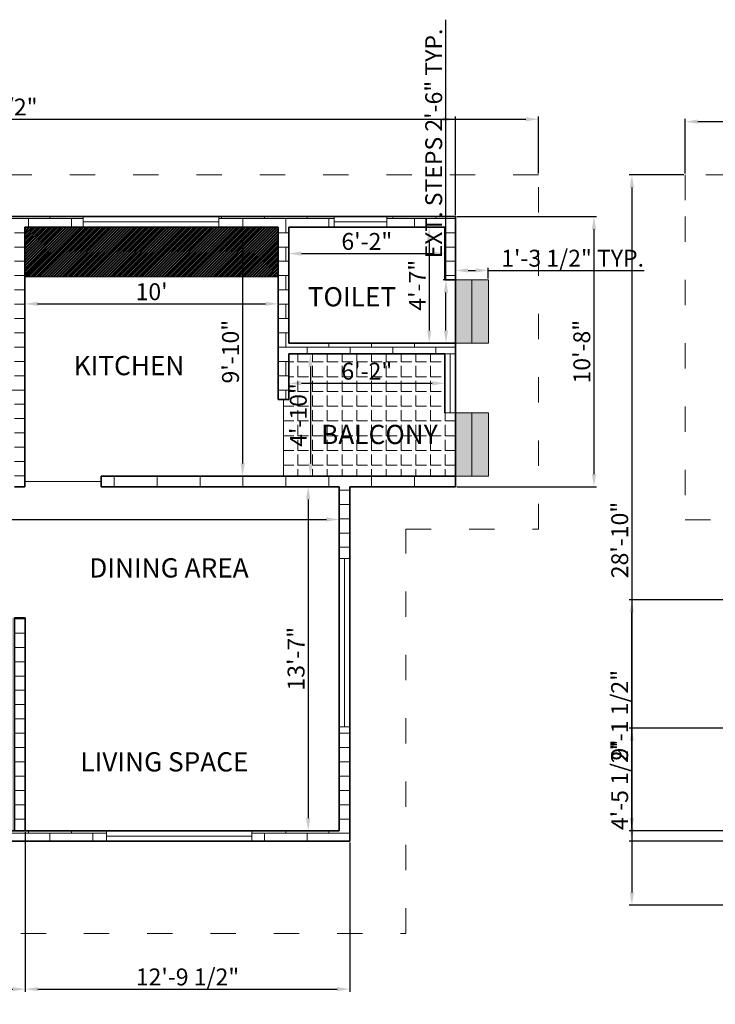
# Model space of a CAD drawing. Units: millimetres. Extents: x 1518 to 2850, y 936 to 2174.
# Tile 3 of 5: x 2007 to 2336, y 1707 to 2174. Entities that reach past the tile are written whole.
import ezdxf

# ---------------------------------------------------------------- set-up
doc = ezdxf.new("R2010")
doc.units = ezdxf.units.MM
doc.linetypes.add('ACAD_ISO03W100', pattern=[30, 12, -18])
for name, color, linetype, lineweight, true_color in [('A-ANNO-DIMS', 9, 'Continuous', 18, 0xafd9aa), ('A-AREA-IDEN', 31, 'Continuous', 18, 0xfecc66), ('A-DOOR', 244, 'Continuous', 20, 0x991b1e), ('A-FLOR-FIXT-PATT', 254, 'Continuous', 13, 0xfeeab9), ('A-FLOR-PATT', 252, 'Continuous', 13, 0x939598), ('A-GLAZ', 141, 'Continuous', 18, 0xadddf7), ('A-ROOF-OVHD', 177, 'ACAD_ISO03W100', 18, 0x293189)]:
    doc.layers.add(name, color=color, linetype=linetype, lineweight=lineweight, true_color=true_color)
for name, color, linetype, lineweight in [('A-FLOR-FIXT', 8, 'Continuous', 18), ('A-FLOR-STRS', 7, 'Continuous', 20), ('A-FLOR-STRS-PATT', 7, 'Continuous', 13), ('A-WALL', 7, 'Continuous', 35), ('A-WALL-PATT', 7, 'Continuous', 13)]:
    doc.layers.add(name, color=color, linetype=linetype, lineweight=lineweight)
doc.styles.get("Standard").update_dxf_attribs({"font": 'arial.ttf'})
doc.dimstyles.new('ISO-25', dxfattribs={"dimtxt": 8, "dimasz": 6, "dimexe": 1.25, "dimexo": 0.625, "dimtad": 1, "dimdec": 0, "dimlunit": 3, "dimtxsty": 'Standard', "dimcen": 2.5, "dimadec": 0, "dimazin": 0, "dimtfac": 1, "dimtdec": 0, "dimtmove": 0, "dimatfit": 3, "dimfxl": 1, "dimarcsym": 0})

# ---------------------------------------------------------------- blocks, each defined once
blk = doc.blocks.new('*D5')
at = {"layer": 'A-ANNO-DIMS', "color": 0, "lineweight": -2, "transparency": 16777216}
for p, q in [((1790.95, 1951.97), (1790.95, 1935.8)), ((2158.01, 1951.97), (2158.01, 1935.8)), ((1796.95, 1937.05), (2152.01, 1937.05))]:
    blk.add_line(p, q, dxfattribs=at)
at = {"layer": 'A-ANNO-DIMS', "color": 0, "transparency": 16777216}
for points in [[(1796.95, 1938.05), (1796.95, 1936.05), (1790.95, 1937.05)], [(2152.01, 1938.05), (2152.01, 1936.05), (2158.01, 1937.05)]]:
    blk.add_solid(points, dxfattribs=at)
at = {"layer": 'Defpoints', "color": 0, "transparency": 16777216}
for p in [(1790.95, 1952.6), (2158.01, 1952.6), (2158.01, 1937.05)]:
    blk.add_point(p, dxfattribs=at)
at = {"layer": 'A-ANNO-DIMS', "color": 0, "transparency": 16777216, "insert": (1974.48, 1941.76), "char_height": 8, "attachment_point": 5}
blk.add_mtext('30\'-7"', dxfattribs=at)
blk = doc.blocks.new('*D7')
at = {"layer": 'A-ANNO-DIMS', "color": 0, "lineweight": -2, "transparency": 16777216}
for p, q in [((2009.13, 2074.9), (2009.13, 2037.95)), ((2129.13, 2074.9), (2129.13, 2037.95)), ((2015.13, 2039.2), (2123.13, 2039.2))]:
    blk.add_line(p, q, dxfattribs=at)
at = {"layer": 'A-ANNO-DIMS', "color": 0, "transparency": 16777216}
for points in [[(2015.13, 2040.2), (2015.13, 2038.2), (2009.13, 2039.2)], [(2123.13, 2040.2), (2123.13, 2038.2), (2129.13, 2039.2)]]:
    blk.add_solid(points, dxfattribs=at)
at = {"layer": 'Defpoints', "color": 0, "transparency": 16777216}
for p in [(2009.13, 2075.52), (2129.13, 2075.52), (2129.13, 2039.2)]:
    blk.add_point(p, dxfattribs=at)
at = {"layer": 'A-ANNO-DIMS', "color": 0, "transparency": 16777216, "insert": (2069.13, 2043.91), "char_height": 8, "attachment_point": 5}
blk.add_mtext("10'", dxfattribs=at)
blk = doc.blocks.new('*D8')
at = {"layer": 'A-ANNO-DIMS', "color": 0, "lineweight": -2, "transparency": 16777216}
for p, q in [((2128.5, 2075.52), (2111.02, 2075.52)), ((2112.27, 2069.52), (2112.27, 1963.6)), ((2128.5, 1957.6), (2111.02, 1957.6))]:
    blk.add_line(p, q, dxfattribs=at)
at = {"layer": 'A-ANNO-DIMS', "color": 0, "transparency": 16777216}
for points in [[(2111.27, 2069.52), (2113.27, 2069.52), (2112.27, 2075.52)], [(2111.27, 1963.6), (2113.27, 1963.6), (2112.27, 1957.6)]]:
    blk.add_solid(points, dxfattribs=at)
at = {"layer": 'Defpoints', "color": 0, "transparency": 16777216}
for p in [(2129.13, 2075.52), (2112.27, 1957.6), (2129.13, 1957.6)]:
    blk.add_point(p, dxfattribs=at)
at = {"layer": 'A-ANNO-DIMS', "color": 0, "transparency": 16777216, "insert": (2107.56, 2016.56), "char_height": 8, "attachment_point": 5, "rotation": 90}
blk.add_mtext('9\'-10"', dxfattribs=at)
blk = doc.blocks.new('*D9')
at = {"layer": 'A-ANNO-DIMS', "color": 0, "lineweight": -2, "transparency": 16777216}
for p, q in [((2134.13, 2074.9), (2134.13, 2061.77)), ((2208.13, 2074.9), (2208.13, 2061.77)), ((2140.13, 2063.02), (2202.13, 2063.02))]:
    blk.add_line(p, q, dxfattribs=at)
at = {"layer": 'A-ANNO-DIMS', "color": 0, "transparency": 16777216}
for points in [[(2140.13, 2064.02), (2140.13, 2062.02), (2134.13, 2063.02)], [(2202.13, 2064.02), (2202.13, 2062.02), (2208.13, 2063.02)]]:
    blk.add_solid(points, dxfattribs=at)
at = {"layer": 'Defpoints', "color": 0, "transparency": 16777216}
for p in [(2134.13, 2075.52), (2208.13, 2075.52), (2208.13, 2063.02)]:
    blk.add_point(p, dxfattribs=at)
at = {"layer": 'A-ANNO-DIMS', "color": 0, "transparency": 16777216, "insert": (2171.13, 2067.73), "char_height": 8, "attachment_point": 5}
blk.add_mtext('6\'-2"', dxfattribs=at)
blk = doc.blocks.new('*D10')
at = {"layer": 'A-ANNO-DIMS', "color": 0, "lineweight": -2, "transparency": 16777216}
for p, q in [((2207.5, 2075.52), (2199.46, 2075.52)), ((2200.71, 2069.52), (2200.71, 2026.52)), ((2207.5, 2020.52), (2199.46, 2020.52))]:
    blk.add_line(p, q, dxfattribs=at)
at = {"layer": 'A-ANNO-DIMS', "color": 0, "transparency": 16777216}
for points in [[(2199.71, 2069.52), (2201.71, 2069.52), (2200.71, 2075.52)], [(2199.71, 2026.52), (2201.71, 2026.52), (2200.71, 2020.52)]]:
    blk.add_solid(points, dxfattribs=at)
at = {"layer": 'Defpoints', "color": 0, "transparency": 16777216}
for p in [(2208.13, 2075.52), (2200.71, 2020.52), (2208.13, 2020.52)]:
    blk.add_point(p, dxfattribs=at)
at = {"layer": 'A-ANNO-DIMS', "color": 0, "transparency": 16777216, "insert": (2196.09, 2048.02), "char_height": 8, "attachment_point": 5, "rotation": 90}
blk.add_mtext('4\'-7"', dxfattribs=at)
blk = doc.blocks.new('*D11')
at = {"layer": 'A-ANNO-DIMS', "color": 0, "lineweight": -2, "transparency": 16777216}
for p, q in [((2134.75, 2015.52), (2145.64, 2015.52)), ((2144.39, 2009.52), (2144.39, 1963.6)), ((2134.75, 1957.6), (2145.64, 1957.6))]:
    blk.add_line(p, q, dxfattribs=at)
at = {"layer": 'A-ANNO-DIMS', "color": 0, "transparency": 16777216}
for points in [[(2143.39, 2009.52), (2145.39, 2009.52), (2144.39, 2015.52)], [(2143.39, 1963.6), (2145.39, 1963.6), (2144.39, 1957.6)]]:
    blk.add_solid(points, dxfattribs=at)
at = {"layer": 'Defpoints', "color": 0, "transparency": 16777216}
for p in [(2134.13, 2015.52), (2134.13, 1957.6), (2144.39, 1957.6)]:
    blk.add_point(p, dxfattribs=at)
at = {"layer": 'A-ANNO-DIMS', "color": 0, "transparency": 16777216, "insert": (2139.68, 1986.56), "char_height": 8, "attachment_point": 5, "rotation": 90}
blk.add_mtext('4\'-10"', dxfattribs=at)
blk = doc.blocks.new('*D12')
at = {"layer": 'A-ANNO-DIMS', "color": 0, "lineweight": -2, "transparency": 16777216}
for p, q in [((2134.13, 2014.9), (2134.13, 2000.31)), ((2208.13, 2014.9), (2208.13, 2000.31)), ((2140.13, 2001.56), (2202.13, 2001.56))]:
    blk.add_line(p, q, dxfattribs=at)
at = {"layer": 'A-ANNO-DIMS', "color": 0, "transparency": 16777216}
for points in [[(2140.13, 2002.56), (2140.13, 2000.56), (2134.13, 2001.56)], [(2202.13, 2002.56), (2202.13, 2000.56), (2208.13, 2001.56)]]:
    blk.add_solid(points, dxfattribs=at)
at = {"layer": 'Defpoints', "color": 0, "transparency": 16777216}
for p in [(2134.13, 2015.52), (2208.13, 2015.52), (2208.13, 2001.56)]:
    blk.add_point(p, dxfattribs=at)
at = {"layer": 'A-ANNO-DIMS', "color": 0, "transparency": 16777216, "insert": (2171.13, 2006.27), "char_height": 8, "attachment_point": 5}
blk.add_mtext('6\'-2"', dxfattribs=at)
blk = doc.blocks.new('*D13')
at = {"layer": 'A-ANNO-DIMS', "color": 0, "lineweight": -2, "transparency": 16777216}
for p, q in [((2157.38, 1952.6), (2142.09, 1952.6)), ((2143.34, 1946.6), (2143.34, 1795.6)), ((2157.38, 1789.6), (2142.09, 1789.6))]:
    blk.add_line(p, q, dxfattribs=at)
at = {"layer": 'A-ANNO-DIMS', "color": 0, "transparency": 16777216}
for points in [[(2142.34, 1946.6), (2144.34, 1946.6), (2143.34, 1952.6)], [(2142.34, 1795.6), (2144.34, 1795.6), (2143.34, 1789.6)]]:
    blk.add_solid(points, dxfattribs=at)
at = {"layer": 'Defpoints', "color": 0, "transparency": 16777216}
for p in [(2158.01, 1952.6), (2143.34, 1789.6), (2158.01, 1789.6)]:
    blk.add_point(p, dxfattribs=at)
at = {"layer": 'A-ANNO-DIMS', "color": 0, "transparency": 16777216, "insert": (2138.63, 1871.1), "char_height": 8, "attachment_point": 5, "rotation": 90}
blk.add_mtext('13\'-7"', dxfattribs=at)
blk = doc.blocks.new('STEP-PAIR-EXT')
for points in [[(0, 30), (7.79, 30), (7.79, 0), (0, 0)], [(7.79, 30), (15.58, 30), (15.58, 0), (7.79, 0)]]:
    blk.add_lwpolyline(points, close=True)
blk = doc.blocks.new('*D28')
at = {"layer": 'A-ANNO-DIMS', "color": 0, "lineweight": -2, "transparency": 16777216}
for p, q in [((2208.63, 2050.52), (2208.63, 2173.81)), ((2212.5, 2050.52), (2207.38, 2050.52)), ((2208.63, 2026.52), (2208.63, 2044.52)), ((2212.5, 2020.52), (2207.38, 2020.52))]:
    blk.add_line(p, q, dxfattribs=at)
at = {"layer": 'A-ANNO-DIMS', "color": 0, "transparency": 16777216}
for points in [[(2207.63, 2044.52), (2209.63, 2044.52), (2208.63, 2050.52)], [(2207.63, 2026.52), (2209.63, 2026.52), (2208.63, 2020.52)]]:
    blk.add_solid(points, dxfattribs=at)
at = {"layer": 'Defpoints', "color": 0, "transparency": 16777216}
for p in [(2208.63, 2050.52), (2213.13, 2050.52), (2213.13, 2020.52)]:
    blk.add_point(p, dxfattribs=at)
at = {"layer": 'A-ANNO-DIMS', "color": 0, "transparency": 16777216, "insert": (2203.86, 2115.17), "char_height": 8, "attachment_point": 5, "rotation": 90}
blk.add_mtext('EXT. STEPS 2\'-6" TYP.', dxfattribs=at)
blk = doc.blocks.new('*D29')
at = {"layer": 'A-ANNO-DIMS', "color": 0, "lineweight": -2, "transparency": 16777216}
for p, q in [((2213.13, 2051.15), (2213.13, 2056.27)), ((2219.13, 2055.02), (2222.7, 2055.02)), ((2228.7, 2051.15), (2228.7, 2056.27)), ((2228.7, 2055.02), (2302.6, 2055.02))]:
    blk.add_line(p, q, dxfattribs=at)
at = {"layer": 'A-ANNO-DIMS', "color": 0, "transparency": 16777216}
for points in [[(2219.13, 2056.02), (2219.13, 2054.02), (2213.13, 2055.02)], [(2222.7, 2056.02), (2222.7, 2054.02), (2228.7, 2055.02)]]:
    blk.add_solid(points, dxfattribs=at)
at = {"layer": 'Defpoints', "color": 0, "transparency": 16777216}
for p in [(2228.7, 2055.02), (2213.13, 2050.52), (2228.7, 2050.52)]:
    blk.add_point(p, dxfattribs=at)
at = {"layer": 'A-ANNO-DIMS', "color": 0, "transparency": 16777216, "insert": (2268.65, 2059.79), "char_height": 8, "attachment_point": 5}
blk.add_mtext('1\'-3 1/2" TYP.', dxfattribs=at)
blk = doc.blocks.new('*D32')
at = {"layer": 'A-ANNO-DIMS', "color": 0, "lineweight": -2, "transparency": 16777216}
for p, q in [((1750, 2081.15), (1750, 2127.88)), ((2213.13, 2081.15), (2213.13, 2127.88)), ((1756, 2126.63), (2207.13, 2126.63))]:
    blk.add_line(p, q, dxfattribs=at)
at = {"layer": 'A-ANNO-DIMS', "color": 0, "transparency": 16777216}
for points in [[(1756, 2127.63), (1756, 2125.63), (1750, 2126.63)], [(2207.13, 2127.63), (2207.13, 2125.63), (2213.13, 2126.63)]]:
    blk.add_solid(points, dxfattribs=at)
at = {"layer": 'Defpoints', "color": 0, "transparency": 16777216}
for p in [(2213.13, 2126.63), (1750, 2080.52), (2213.13, 2080.52)]:
    blk.add_point(p, dxfattribs=at)
at = {"layer": 'A-ANNO-DIMS', "color": 0, "transparency": 16777216, "insert": (1981.56, 2131.34), "char_height": 8, "attachment_point": 5}
blk.add_mtext('38\'-7"', dxfattribs=at)
blk = doc.blocks.new('*D33')
at = {"layer": 'A-ANNO-DIMS', "color": 0, "lineweight": -2, "transparency": 16777216}
for p, q in [((2213.75, 2080.52), (2280, 2080.52)), ((2278.75, 2074.52), (2278.75, 1958.6)), ((2213.75, 1952.6), (2280, 1952.6))]:
    blk.add_line(p, q, dxfattribs=at)
at = {"layer": 'A-ANNO-DIMS', "color": 0, "transparency": 16777216}
for points in [[(2277.75, 2074.52), (2279.75, 2074.52), (2278.75, 2080.52)], [(2277.75, 1958.6), (2279.75, 1958.6), (2278.75, 1952.6)]]:
    blk.add_solid(points, dxfattribs=at)
at = {"layer": 'Defpoints', "color": 0, "transparency": 16777216}
for p in [(2213.13, 2080.52), (2213.13, 1952.6), (2278.75, 1952.6)]:
    blk.add_point(p, dxfattribs=at)
at = {"layer": 'A-ANNO-DIMS', "color": 0, "transparency": 16777216, "insert": (2274.04, 2016.56), "char_height": 8, "attachment_point": 5, "rotation": 90}
blk.add_mtext('10\'-8"', dxfattribs=at)
blk = doc.blocks.new('*D36')
at = {"layer": 'A-ANNO-DIMS', "color": 0, "lineweight": -2, "transparency": 16777216}
for p, q in [((2009.3, 1788.97), (2009.3, 1713.31)), ((1909.3, 1783.97), (1909.3, 1713.31)), ((1915.3, 1714.56), (2003.3, 1714.56))]:
    blk.add_line(p, q, dxfattribs=at)
at = {"layer": 'A-ANNO-DIMS', "color": 0, "transparency": 16777216}
for points in [[(1915.3, 1715.56), (1915.3, 1713.56), (1909.3, 1714.56)], [(2003.3, 1715.56), (2003.3, 1713.56), (2009.3, 1714.56)]]:
    blk.add_solid(points, dxfattribs=at)
at = {"layer": 'Defpoints', "color": 0, "transparency": 16777216}
for p in [(2009.3, 1789.6), (1909.3, 1784.6), (2009.3, 1714.56)]:
    blk.add_point(p, dxfattribs=at)
at = {"layer": 'A-ANNO-DIMS', "color": 0, "transparency": 16777216, "insert": (1959.3, 1719.27), "char_height": 8, "attachment_point": 5}
blk.add_mtext('8\'-4"', dxfattribs=at)
blk = doc.blocks.new('*D37')
at = {"layer": 'A-ANNO-DIMS', "color": 0, "lineweight": -2, "transparency": 16777216}
for p, q in [((2009.3, 1788.97), (2009.3, 1713.31)), ((2163.01, 1783.97), (2163.01, 1713.31)), ((2015.3, 1714.56), (2157.01, 1714.56))]:
    blk.add_line(p, q, dxfattribs=at)
at = {"layer": 'A-ANNO-DIMS', "color": 0, "transparency": 16777216}
for points in [[(2015.3, 1715.56), (2015.3, 1713.56), (2009.3, 1714.56)], [(2157.01, 1715.56), (2157.01, 1713.56), (2163.01, 1714.56)]]:
    blk.add_solid(points, dxfattribs=at)
at = {"layer": 'Defpoints', "color": 0, "transparency": 16777216}
for p in [(2009.3, 1789.6), (2163.01, 1784.6), (2163.01, 1714.56)]:
    blk.add_point(p, dxfattribs=at)
at = {"layer": 'A-ANNO-DIMS', "color": 0, "transparency": 16777216, "insert": (2086.16, 1719.32), "char_height": 8, "attachment_point": 5}
blk.add_mtext('12\'-9 1/2"', dxfattribs=at)
blk = doc.blocks.new('*D40')
at = {"layer": 'A-ANNO-DIMS', "color": 0, "lineweight": -2, "transparency": 16777216}
for p, q in [((1728.79, 2100.9), (1728.79, 2127.88)), ((2252.4, 2100.9), (2252.4, 2127.88)), ((1734.79, 2126.63), (2246.4, 2126.63))]:
    blk.add_line(p, q, dxfattribs=at)
at = {"layer": 'A-ANNO-DIMS', "color": 0, "transparency": 16777216}
for points in [[(1734.79, 2127.63), (1734.79, 2125.63), (1728.79, 2126.63)], [(2246.4, 2127.63), (2246.4, 2125.63), (2252.4, 2126.63)]]:
    blk.add_solid(points, dxfattribs=at)
at = {"layer": 'Defpoints', "color": 0, "transparency": 16777216}
for p in [(2252.4, 2126.63), (1728.79, 2100.28), (2252.4, 2100.28)]:
    blk.add_point(p, dxfattribs=at)
at = {"layer": 'A-ANNO-DIMS', "color": 0, "transparency": 16777216, "insert": (1990.6, 2131.39), "char_height": 8, "attachment_point": 5}
blk.add_mtext('43\'-7 1/2"', dxfattribs=at)
blk = doc.blocks.new('*D48')
at = {"layer": 'A-ANNO-DIMS', "color": 0, "lineweight": -2, "transparency": 16777216}
for p, q in [((2588.86, 1899.05), (2295.47, 1899.05)), ((2296.72, 1795.6), (2296.72, 1893.05)), ((2588.86, 1789.6), (2295.47, 1789.6))]:
    blk.add_line(p, q, dxfattribs=at)
at = {"layer": 'A-ANNO-DIMS', "color": 0, "transparency": 16777216}
for points in [[(2295.72, 1893.05), (2297.72, 1893.05), (2296.72, 1899.05)], [(2295.72, 1795.6), (2297.72, 1795.6), (2296.72, 1789.6)]]:
    blk.add_solid(points, dxfattribs=at)
at = {"layer": 'Defpoints', "color": 0, "transparency": 16777216}
for p in [(2296.72, 1899.05), (2589.49, 1899.05), (2589.49, 1789.6)]:
    blk.add_point(p, dxfattribs=at)
at = {"layer": 'A-ANNO-DIMS', "color": 0, "transparency": 16777216, "insert": (2291.96, 1844.32), "char_height": 8, "attachment_point": 5, "rotation": 90}
blk.add_mtext('9\'-1 1/2"', dxfattribs=at)
blk = doc.blocks.new('*D49')
at = {"layer": 'A-ANNO-DIMS', "color": 0, "lineweight": -2, "transparency": 16777216}
for p, q in [((2363.13, 1838.2), (2295.47, 1838.2)), ((2296.72, 1790.6), (2296.72, 1832.2)), ((2363.13, 1784.6), (2295.47, 1784.6))]:
    blk.add_line(p, q, dxfattribs=at)
at = {"layer": 'A-ANNO-DIMS', "color": 0, "transparency": 16777216}
for points in [[(2295.72, 1832.2), (2297.72, 1832.2), (2296.72, 1838.2)], [(2295.72, 1790.6), (2297.72, 1790.6), (2296.72, 1784.6)]]:
    blk.add_solid(points, dxfattribs=at)
at = {"layer": 'Defpoints', "color": 0, "transparency": 16777216}
for p in [(2296.72, 1838.2), (2363.76, 1838.2), (2363.76, 1784.6)]:
    blk.add_point(p, dxfattribs=at)
at = {"layer": 'A-ANNO-DIMS', "color": 0, "transparency": 16777216, "insert": (2291.96, 1811.4), "char_height": 8, "attachment_point": 5, "rotation": 90}
blk.add_mtext('4\'-5 1/2"', dxfattribs=at)
blk = doc.blocks.new('*D50')
at = {"layer": 'A-ANNO-DIMS', "color": 0, "lineweight": -2, "transparency": 16777216}
for p, q in [((2321.97, 2100.9), (2321.97, 2126.78)), ((2327.97, 2125.53), (2817.73, 2125.53)), ((2823.73, 2100.9), (2823.73, 2126.78))]:
    blk.add_line(p, q, dxfattribs=at)
at = {"layer": 'A-ANNO-DIMS', "color": 0, "transparency": 16777216}
for points in [[(2327.97, 2126.53), (2327.97, 2124.53), (2321.97, 2125.53)], [(2817.73, 2126.53), (2817.73, 2124.53), (2823.73, 2125.53)]]:
    blk.add_solid(points, dxfattribs=at)
at = {"layer": 'Defpoints', "color": 0, "transparency": 16777216}
for p in [(2823.73, 2125.53), (2321.97, 2100.28), (2823.73, 2100.28)]:
    blk.add_point(p, dxfattribs=at)
at = {"layer": 'A-ANNO-DIMS', "color": 0, "transparency": 16777216, "insert": (2572.85, 2130.24), "char_height": 8, "attachment_point": 5}
blk.add_mtext('41\'-10"', dxfattribs=at)
blk = doc.blocks.new('*D51')
at = {"layer": 'A-ANNO-DIMS', "color": 0, "lineweight": -2, "transparency": 16777216}
for p, q in [((2321.34, 2100.28), (2295.47, 2100.28)), ((2296.72, 2094.28), (2296.72, 1760.39)), ((2347.23, 1754.39), (2295.47, 1754.39))]:
    blk.add_line(p, q, dxfattribs=at)
at = {"layer": 'A-ANNO-DIMS', "color": 0, "transparency": 16777216}
for points in [[(2295.72, 2094.28), (2297.72, 2094.28), (2296.72, 2100.28)], [(2295.72, 1760.39), (2297.72, 1760.39), (2296.72, 1754.39)]]:
    blk.add_solid(points, dxfattribs=at)
at = {"layer": 'Defpoints', "color": 0, "transparency": 16777216}
for p in [(2321.97, 2100.28), (2296.72, 1754.39), (2347.86, 1754.39)]:
    blk.add_point(p, dxfattribs=at)
at = {"layer": 'A-ANNO-DIMS', "color": 0, "transparency": 16777216, "insert": (2292.01, 1927.34), "char_height": 8, "attachment_point": 5, "rotation": 90}
blk.add_mtext('28\'-10"', dxfattribs=at)

msp = doc.modelspace()

# ---------------------------------------------------------------- hatches: boundary and pattern name
at = {"layer": 'A-FLOR-FIXT-PATT'}
h = msp.add_hatch(dxfattribs=at)
h.set_pattern_fill('ANSI32', color=256, scale=0.1)
h.set_pattern_definition([(45, (-61.8398, 0), (-0.6735192, 0.6735192), []), (45, (-61.3908, 0), (-0.6735192, 0.6735192), [])])
h.paths.add_polyline_path([(2009.13, 2075.52), (2009.13, 2052.02), (2129.13, 2052.02), (2129.13, 2075.52)])
at = {"layer": 'A-FLOR-PATT'}
h = msp.add_hatch(dxfattribs=at)
h.set_pattern_fill('ANGLE', color=256)
h.set_pattern_definition([(0, (-61.84, 0), (0, 6.985), [5.08, -1.905]), (90, (-61.84, 0), (-6.985, 4e-16), [5.08, -1.905])])
h.paths.add_polyline_path([(1909.3, 1784.6), (1909.3, 1838.2), (1909.3, 1840.7), (1872.42, 1840.7), (1872.42, 1838.2), (1785.95, 1838.2), (1785.95, 1784.62)])
h.paths.add_polyline_path([(2134.13, 2015.52), (2134.13, 1993.83), (2131.63, 1993.83), (2131.63, 1957.6), (2134.13, 1957.6), (2208.13, 1957.6), (2213.13, 1957.6), (2213.13, 1987.59), (2208.13, 1987.59), (2208.13, 2015.52)])
at = {"layer": 'A-FLOR-STRS-PATT'}
h = msp.add_hatch(dxfattribs=at)
h.set_pattern_fill('AR-RROOF', color=256, scale=0.1)
h.set_pattern_definition([(0, (-61.8398, 0), (5.588, 2.54), [38.1, -5.08, 12.7, -2.54]), (0, (-58.4616, 1.27), (-2.54, 3.3782), [7.62, -0.8382, 15.24, -1.905]), (0, (-60.5698, 2.159), (13.208, 1.7018), [20.32, -3.556, 10.16, -2.54])])
h.paths.add_polyline_path([(1909.3, 1784.6), (1785.95, 1784.62), (1785.95, 1772.51), (1909.3, 1772.51)])
h.paths.add_polyline_path([(1909.3, 1772.51), (1785.95, 1772.51), (1785.95, 1760.21), (1909.3, 1760.21)])
h.paths.add_polyline_path([(2004.13, 1830.49), (1959.21, 1830.49), (1959.21, 1818.49), (2004.13, 1818.49)])
h.paths.add_polyline_path([(2004.13, 1818.49), (1959.21, 1818.49), (1914.3, 1818.49), (1914.3, 1789.6), (2004.13, 1789.6)])
h.paths.add_polyline_path([(1959.21, 1830.49), (1914.3, 1830.49), (1914.3, 1818.49), (1959.21, 1818.49)])
h.paths.add_polyline_path([(1959.21, 1842.49), (1914.3, 1842.49), (1914.3, 1830.49), (1959.21, 1830.49)])
h.paths.add_polyline_path([(1959.21, 1854.49), (1914.3, 1854.49), (1914.3, 1842.49), (1959.21, 1842.49)])
h.paths.add_polyline_path([(1959.21, 1866.49), (1914.3, 1866.49), (1914.3, 1854.49), (1959.21, 1854.49)])
h.paths.add_polyline_path([(2004.13, 1890.49), (1959.21, 1890.49), (1959.21, 1878.49), (2004.13, 1878.49)])
h.paths.add_polyline_path([(2004.13, 1878.49), (1959.21, 1878.49), (1959.21, 1866.49), (2004.13, 1866.49)])
h.paths.add_polyline_path([(2004.13, 1866.49), (1959.21, 1866.49), (1959.21, 1854.49), (2004.13, 1854.49)])
h.paths.add_polyline_path([(2004.13, 1854.49), (1959.21, 1854.49), (1959.21, 1842.49), (2004.13, 1842.49)])
h.paths.add_polyline_path([(2004.13, 1842.49), (1959.21, 1842.49), (1959.21, 1830.49), (2004.13, 1830.49)])
h.paths.add_polyline_path([(2228.7, 1987.6), (2220.91, 1987.6), (2220.91, 1957.6), (2228.7, 1957.6)])
h.paths.add_polyline_path([(2220.91, 1987.6), (2213.13, 1987.6), (2213.13, 1957.6), (2220.91, 1957.6)])
h.paths.add_polyline_path([(2228.7, 2050.52), (2220.91, 2050.52), (2220.91, 2020.52), (2228.7, 2020.52)])
h.paths.add_polyline_path([(2220.91, 2050.52), (2213.13, 2050.52), (2213.13, 2020.52), (2220.91, 2020.52)])
at = {"layer": 'A-WALL-PATT'}
h = msp.add_hatch(dxfattribs=at)
h.set_pattern_fill('AR-BRSTD', color=256, scale=0.1)
h.set_pattern_definition([(0, (-61.84, 0), (0, 6.77418), []), (90, (-61.84, 0), (-10.16, 6.77418), [6.77418, -6.77418])])
h.paths.add_polyline_path([(1750, 1952.6), (1785.95, 1952.6), (1785.95, 1920.45), (1790.95, 1920.45), (1790.95, 1952.6), (1909.3, 1952.6), (1914.3, 1952.6), (1949.13, 1952.6), (1967.34, 1952.6), (1967.34, 1957.6), (1949.13, 1957.6), (1755, 1957.6), (1755, 1992.17), (1750, 1992.17)])
h.paths.add_polyline_path([(1791.93, 2075.52), (1791.93, 2080.52), (1750, 2080.52), (1750, 2045), (1755, 2045), (1755, 2075.52)])
h.paths.add_polyline_path([(1944.13, 2075.52), (1949.13, 2075.52), (1958.76, 2075.52), (1958.76, 2080.52), (1949.13, 2080.52), (1840.29, 2080.52), (1840.29, 2075.52)])
h.paths.add_polyline_path([(2004.13, 2075.52), (2004.13, 2001.52), (1949.13, 2001.52), (1949.13, 2036.02), (1944.13, 2036.02), (1944.13, 1996.52), (1949.13, 1996.52), (2004.13, 1996.52), (2004.13, 1957.6), (2004.13, 1952.6), (2009.13, 1952.6), (2009.13, 1957.6), (2009.13, 1996.52), (2009.13, 2075.52), (2036.64, 2075.52), (2036.64, 2080.52), (2009.13, 2080.52), (1995.08, 2080.52), (1995.08, 2075.52)])
h.paths.add_polyline_path([(2101.06, 2080.52), (2101.06, 2075.52), (2129.13, 2075.52), (2129.13, 1993.83), (2134.13, 1993.83), (2134.13, 2015.52), (2208.13, 2015.52), (2213.13, 2015.52), (2213.13, 2020.52), (2208.13, 2020.52), (2134.13, 2020.52), (2134.13, 2075.52), (2155.67, 2075.52), (2155.67, 2080.52), (2129.13, 2080.52)])
h.paths.add_polyline_path([(2180.68, 2080.52), (2180.68, 2075.52), (2208.13, 2075.52), (2208.13, 2050.52), (2213.13, 2050.52), (2213.13, 2080.52)], flags=17)
h.paths.add_polyline_path([(2129.13, 1952.6), (2158.01, 1952.6), (2158.01, 1918.63), (2163.01, 1918.63), (2163.01, 1952.6), (2213.13, 1952.6), (2213.13, 1957.6), (2208.13, 1957.6), (2134.13, 1957.6), (2129.13, 1957.6), (2045.26, 1957.6), (2045.26, 1952.6)])
h.paths.add_polyline_path([(2116.7, 1789.6), (2116.7, 1784.6), (2163.01, 1784.6), (2163.01, 1838.76), (2158.01, 1838.76), (2158.01, 1789.6)])
h.paths.add_polyline_path([(2047.7, 1784.6), (2047.7, 1789.6), (1981.4, 1789.6), (1981.4, 1784.6)])
h.paths.add_polyline_path([(2009.3, 1890.49), (2004.13, 1890.49), (2004.13, 1789.6), (2009.3, 1789.6)])
h.paths.add_polyline_path([(1930.65, 1784.6), (1930.65, 1789.6), (1914.3, 1789.6), (1914.3, 1887.35), (1909.3, 1887.35), (1909.3, 1843.2), (1909.3, 1838.2), (1909.3, 1784.6)])
h.paths.add_polyline_path([(1872.42, 1838.2), (1872.42, 1843.2), (1843.67, 1843.2), (1843.67, 1838.2)])
h.paths.add_polyline_path([(1790.95, 1843.2), (1790.95, 1879.12), (1785.95, 1879.12), (1785.95, 1838.2), (1806.76, 1838.2), (1806.76, 1843.2)])

# ---------------------------------------------------------------- linework, layer by layer
at = {"layer": 'A-DOOR'}
for p, q in [((2131.63, 1993.83), (2131.63, 1957.6)), ((2045.26, 1955.1), (2009.13, 1955.1))]:
    msp.add_line(p, q, dxfattribs=at)
at = {"layer": 'A-FLOR-FIXT'}
msp.add_line((2009.13, 2052.02), (2129.13, 2052.02), dxfattribs=at)
at = {"layer": 'A-GLAZ'}
for p, q in [((2036.64, 2078.02), (2101.06, 2078.02)), ((2155.67, 2078.02), (2180.68, 2078.02)), ((2210.63, 2015.52), (2210.63, 1987.59)), ((2160.51, 1918.63), (2160.51, 1838.76)), ((2047.7, 1787.1), (2116.7, 1787.1))]:
    msp.add_line(p, q, dxfattribs=at)
for points in [[(2036.64, 2080.52), (2101.06, 2080.52), (2101.06, 2075.52), (2036.64, 2075.52)], [(2155.67, 2080.52), (2180.68, 2080.52), (2180.68, 2075.52), (2155.67, 2075.52)], [(2208.13, 2015.52), (2213.13, 2015.52), (2213.13, 1987.59), (2208.13, 1987.59)], [(2163.01, 1918.63), (2158.01, 1918.63), (2158.01, 1838.76), (2163.01, 1838.76)], [(2047.7, 1789.6), (2116.7, 1789.6), (2116.7, 1784.6), (2047.7, 1784.6)]]:
    msp.add_lwpolyline(points, close=True, dxfattribs=at)
at = {"layer": 'A-ROOF-OVHD'}
for p, q in [((2252.4, 2100.28), (1728.79, 2100.28)), ((2252.4, 1932.53), (2252.4, 2100.28)), ((2823.73, 2100.28), (2321.97, 2100.28)), ((2321.97, 2100.28), (2321.97, 2080.52)), ((2321.97, 2080.52), (2321.97, 1936.95)), ((2321.97, 1936.95), (2347.86, 1936.95)), ((2189.67, 1740.91), (2189.67, 1932.53)), ((2189.67, 1932.53), (2252.4, 1932.53)), ((1767.1, 1740.91), (2189.67, 1740.91))]:
    msp.add_line(p, q, dxfattribs=at)
at = {"layer": 'A-WALL'}
for p, q in [((1949.13, 2080.52), (2009.13, 2080.52)), ((2009.13, 2080.52), (2129.13, 2080.52)), ((2129.13, 2080.52), (2213.13, 2080.52)), ((2213.13, 2080.52), (2213.13, 2020.52)), ((2009.13, 2075.52), (2009.13, 1996.52)), ((2009.13, 2075.52), (2129.13, 2075.52)), ((2129.13, 2075.52), (2129.13, 1993.83)), ((2134.13, 2075.52), (2208.13, 2075.52)), ((2134.13, 2075.52), (2134.13, 2020.52)), ((2208.13, 2075.52), (2208.13, 2050.52)), ((2208.13, 2020.52), (2134.13, 2020.52)), ((2213.13, 2020.52), (2213.13, 1952.6)), ((2208.13, 2015.52), (2134.13, 2015.52)), ((2134.13, 2015.52), (2134.13, 1993.83)), ((2208.13, 2015.52), (2208.13, 1987.59)), ((2009.13, 1957.6), (2009.13, 1996.52)), ((2129.13, 1957.6), (2045.26, 1957.6)), ((2208.13, 1957.6), (2134.13, 1957.6)), ((2004.13, 1952.6), (2009.13, 1952.6)), ((2129.13, 1952.6), (2045.26, 1952.6)), ((2158.01, 1952.6), (2129.13, 1952.6)), ((2158.01, 1952.6), (2158.01, 1789.6)), ((2213.13, 1952.6), (2163.01, 1952.6)), ((2163.01, 1952.6), (2163.01, 1784.6)), ((2158.01, 1789.6), (1914.3, 1789.6)), ((2163.01, 1784.6), (1909.3, 1784.6))]:
    msp.add_line(p, q, dxfattribs=at)
for points in [[(2208.13, 2020.52), (2213.13, 2020.52), (2213.13, 2050.52), (2208.13, 2050.52)], [(2134.13, 1993.83), (2129.13, 1993.83)], [(2009.13, 1952.6), (2009.13, 1957.6)], [(2045.26, 1957.6), (2045.26, 1952.6)], [(2129.13, 1957.6), (2134.13, 1957.6)], [(2009.3, 1890.49), (2004.13, 1890.49)], [(2009.3, 1890.49), (2009.3, 1789.6), (2004.13, 1789.6), (2004.13, 1890.49)]]:
    msp.add_lwpolyline(points, dxfattribs=at)
msp.add_lwpolyline([(2208.13, 1957.6), (2213.13, 1957.6), (2213.13, 1957.6), (2208.13, 1957.6)], close=True, dxfattribs=at)

# ---------------------------------------------------------------- block references
at = {"layer": 'A-FLOR-STRS'}
for p in [(2213.13, 2020.52), (2213.13, 1957.6)]:
    msp.add_blockref('STEP-PAIR-EXT', p, dxfattribs=at)

# ---------------------------------------------------------------- texts
at = {"layer": 'A-AREA-IDEN'}
for s, height, p in [('TOILET', 9.117, (2143.14, 2038)), ('KITCHEN', 9.117, (2032.22, 2005.39)), ('BALCONY', 9.117, (2149.46, 1972.78)), ('DINING AREA', 9.1171, (2039.59, 1909.56)), ('LIVING SPACE', 9.1171, (2035.38, 1817.69))]:
    msp.add_text(s, height=height, dxfattribs=at).set_placement(p)

# ---------------------------------------------------------------- dimensions: what is measured, and where the dimension line sits
at = {"layer": 'A-ANNO-DIMS'}
dim = msp.add_linear_dim(base=(2208.63, 2050.52), p1=(2213.13, 2020.52), p2=(2213.13, 2050.52), angle=90, text='EXT. STEPS <> TYP.', dimstyle='ISO-25', override={"dimdec": 1, "dimlfac": 1, "dimrnd": 0, "dimzin": 1, "dimdsep": 46, "dimlunit": 4, "dimfrac": 2}, dxfattribs=at)
dim.commit()
dim.dimension.update_dxf_attribs({"geometry": '*D28', "text_midpoint": (2203.86, 2115.17)})
for base, p1, p2, override, picture, middle in [((2252.4, 2126.63), (1728.79, 2100.28), (2252.4, 2100.28), {"dimdec": 1, "dimlfac": 1, "dimrnd": 0, "dimzin": 1, "dimdsep": 46, "dimlunit": 4, "dimfrac": 2}, '*D40', (1990.6, 2131.39)), ((2213.13, 2126.63), (1750, 2080.52), (2213.13, 2080.52), {"dimdec": 1, "dimlfac": 1, "dimrnd": 0, "dimzin": 1, "dimdsep": 46, "dimlunit": 4, "dimfrac": 2}, '*D32', (1981.56, 2131.34)), ((2823.73, 2125.53), (2321.97, 2100.28), (2823.73, 2100.28), {"dimdec": 1, "dimlfac": 1, "dimrnd": 0, "dimzin": 1, "dimdsep": 46, "dimlunit": 4, "dimfrac": 2}, '*D50', (2572.85, 2130.24)), ((2129.13, 2039.2), (2009.13, 2075.52), (2129.13, 2075.52), {"dimclrd": 0, "dimclre": 0, "dimclrt": 0}, '*D7', (2069.13, 2043.91)), ((2208.13, 2063.02), (2134.13, 2075.52), (2208.13, 2075.52), {"dimclrd": 0, "dimclre": 0, "dimclrt": 0}, '*D9', (2171.13, 2067.73)), ((2208.13, 2001.56), (2134.13, 2015.52), (2208.13, 2015.52), {"dimclrd": 0, "dimclre": 0, "dimclrt": 0}, '*D12', (2171.13, 2006.27)), ((2158.01, 1937.05), (1790.95, 1952.6), (2158.01, 1952.6), {"dimclrd": 0, "dimclre": 0, "dimclrt": 0}, '*D5', (1974.48, 1941.76)), ((2009.3, 1714.56), (1909.3, 1784.6), (2009.3, 1789.6), {"dimdec": 1, "dimlfac": 1, "dimrnd": 0, "dimzin": 1, "dimdsep": 46, "dimlunit": 4, "dimfrac": 2}, '*D36', (1959.3, 1719.27)), ((2163.01, 1714.56), (2009.3, 1789.6), (2163.01, 1784.6), {"dimdec": 1, "dimlfac": 1, "dimrnd": 0, "dimzin": 1, "dimdsep": 46, "dimlunit": 4, "dimfrac": 2}, '*D37', (2086.16, 1719.32))]:
    dim = msp.add_linear_dim(base=base, p1=p1, p2=p2, dimstyle='ISO-25', override=override, dxfattribs=at)
    dim.commit()
    dim.dimension.update_dxf_attribs({"geometry": picture, "text_midpoint": middle})
for base, p1, p2, override, picture, middle in [((2296.72, 1754.39), (2321.97, 2100.28), (2347.86, 1754.39), {"dimdec": 1, "dimlfac": 1, "dimrnd": 0, "dimzin": 1, "dimdsep": 46, "dimlunit": 4, "dimfrac": 2}, '*D51', (2292.01, 1927.34)), ((2278.75, 1952.6), (2213.13, 2080.52), (2213.13, 1952.6), {"dimdec": 1, "dimlfac": 1, "dimrnd": 0, "dimzin": 1, "dimdsep": 46, "dimlunit": 4, "dimfrac": 2}, '*D33', (2274.04, 2016.56)), ((2112.27, 1957.6), (2129.13, 2075.52), (2129.13, 1957.6), {"dimclrd": 0, "dimclre": 0, "dimclrt": 0}, '*D8', (2107.56, 2016.56)), ((2200.71, 2020.52), (2208.13, 2075.52), (2208.13, 2020.52), {"dimclrd": 0, "dimclre": 0, "dimclrt": 0}, '*D10', (2196.09, 2048.02)), ((2144.39, 1957.6), (2134.13, 2015.52), (2134.13, 1957.6), {"dimclrd": 0, "dimclre": 0, "dimclrt": 0}, '*D11', (2139.68, 1986.56)), ((2143.34, 1789.6), (2158.01, 1952.6), (2158.01, 1789.6), {"dimclrd": 0, "dimclre": 0, "dimclrt": 0}, '*D13', (2138.63, 1871.1)), ((2296.7185, 1899.0477), (2589.4871, 1789.5976), (2589.4871, 1899.0477), {"dimdec": 1, "dimlfac": 1, "dimrnd": 0, "dimzin": 1, "dimdsep": 46, "dimlunit": 4, "dimfrac": 2}, '*D48', (2291.9571, 1844.3227)), ((2296.72, 1838.2), (2363.76, 1784.6), (2363.76, 1838.2), {"dimdec": 1, "dimlfac": 1, "dimrnd": 0, "dimzin": 1, "dimdsep": 46, "dimlunit": 4, "dimfrac": 2}, '*D49', (2291.96, 1811.4))]:
    dim = msp.add_linear_dim(base=base, p1=p1, p2=p2, angle=90, dimstyle='ISO-25', override=override, dxfattribs=at)
    dim.commit()
    dim.dimension.update_dxf_attribs({"geometry": picture, "text_midpoint": middle})
dim = msp.add_linear_dim(base=(2228.7, 2055.02), p1=(2213.13, 2050.52), p2=(2228.7, 2050.52), text='<> TYP.', dimstyle='ISO-25', override={"dimdec": 1, "dimlfac": 1, "dimrnd": 0, "dimzin": 1, "dimdsep": 46, "dimlunit": 4, "dimfrac": 2}, dxfattribs=at)
dim.commit()
dim.dimension.update_dxf_attribs({"geometry": '*D29', "text_midpoint": (2268.65, 2059.79)})

doc.saveas('drawing.dxf')
